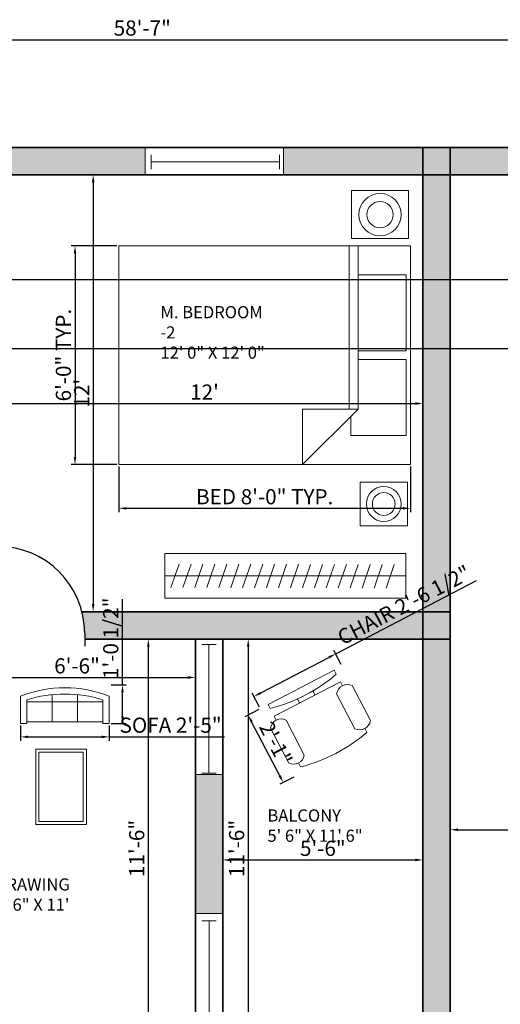
# Model space of a CAD drawing. Units: millimetres. Extents: x 2768 to 4359, y 795 to 1583.
# Tile 12 of 13: x 3930 to 4089, y 1258 to 1583. Entities that reach past the tile are written whole.
import ezdxf

# ---------------------------------------------------------------- set-up
doc = ezdxf.new("R2010")
doc.units = ezdxf.units.MM
for name, color, linetype, lineweight in [('A-ANNO-DIMS', 90, 'Continuous', 18), ('A-AREA-IDEN', 190, 'Continuous', 18), ('A-FLOR-CASE', 50, 'Continuous', 18), ('A-FLOR-CASE-PATT', 50, 'Continuous', 13), ('A-WALL-PATT', 140, 'Continuous', 9), ('doors', 10, 'Continuous', 25), ('furniture', 50, 'Continuous', 18), ('walls', 140, 'Continuous', 35), ('windows', 30, 'Continuous', 18)]:
    doc.layers.add(name, color=color, linetype=linetype, lineweight=lineweight)
doc.styles.get("Standard").update_dxf_attribs({"font": 'arial.ttf'})
doc.dimstyles.new('ISO-25', dxfattribs={"dimtxt": 5, "dimasz": 2.5, "dimexe": 1.25, "dimexo": 0.625, "dimtad": 1, "dimdec": 0, "dimlunit": 3, "dimtxsty": 'Standard', "dimcen": 2.5, "dimadec": 0, "dimazin": 0, "dimtfac": 1, "dimtdec": 0, "dimtmove": 0, "dimatfit": 3, "dimfxl": 1, "dimarcsym": 0})

# ---------------------------------------------------------------- blocks, each defined once
blk = doc.blocks.new('*U2')
for p, q in [((0, 0), (0, -6)), ((40, 0), (40, -6))]:
    blk.add_line(p, q)
blk.add_lwpolyline([(0, 0), (0, 40), (1.75, 40), (1.75, 0)], close=True)
blk.add_arc((0, 0), 40, 0, 90)
blk = doc.blocks.new('*U39')
for p, q in [((0, 4), (0, 0)), ((36, 4), (36, 0)), ((0, 2), (36, 2))]:
    blk.add_line(p, q)
blk = doc.blocks.new('Bed - Queen')
for p, q in [((0, -80.00003), (0, 0)), ((0, 0), (59.99999, 0)), ((59.99999, 0), (59.99999, -80.00003)), ((7.99999, -1.2), (28.79998, -1.2)), ((7.99999, -14.4), (7.99999, -1.2)), ((28.79998, -1.2), (28.79998, -14.4)), ((31.19999, -1.2), (51.99999, -1.2)), ((31.19999, -14.4), (31.19999, -1.2)), ((51.99999, -1.2), (51.99999, -16.4)), ((0, -14.4), (44.8, -14.4)), ((59.99999, -29.6), (44.8, -14.4)), ((44.8, -14.4), (44.8, -29.6)), ((44.8, -16.8), (0, -16.8)), ((51.99999, -16.4), (46.79936, -16.4)), ((44.8, -29.6), (59.99999, -29.6)), ((59.99999, -80.00003), (0, -80.00003))]:
    blk.add_line(p, q)
blk = doc.blocks.new('Chair - Desk')
for p, q in [((-8.5, 0), (-8.5, -1)), ((-8.5, 0), (8.5, 0)), ((8.5, 0), (8.5, -1)), ((-2, -3), (-2, -1.9355)), ((2, -1.9576), (2, -3)), ((-8.5, -3), (-8.5, -4)), ((-8.5, -3), (8.5, -3)), ((8.5, -3), (8.5, -4)), ((-10.5, -5), (-10.5, -14)), ((-6.5, -14), (-6.5, -5)), ((6.5, -5), (6.5, -14)), ((10.5, -14), (10.5, -5)), ((-8.5, -15), (-8.5, -16)), ((8.5, -15), (8.5, -16))]:
    blk.add_line(p, q)
for centre, radius, start, end in [((0, 34.625), 36.625, 256.5803, 283.4197), ((-8.5, -6.5), 2.5, 36.8699, 143.1301), ((8.5, -6.5), 2.5, 36.8699, 143.1301), ((-8.5, -12.5), 2.5, 216.8699, 323.1301), ((8.5, -12.5), 2.5, 216.8699, 323.1301), ((0, 19.625), 36.625, 256.5803, 283.4197)]:
    blk.add_arc(centre, radius, start, end)
blk = doc.blocks.new('Sofa - Roundback 7 ft.')
for p, q in [((-12.00002, -32.4421), (-12.00003, -6.5971)), ((11.99997, -32.4421), (11.99998, -6.5971)), ((-36.000027, -34), (-36.000027, -11.4696)), ((-35.999844, -13.3819), (35.9998, -13.3819)), ((35.99998, -34), (35.99998, -11.4696)), ((-36.000027, -32.4421), (35.99998, -32.4421))]:
    blk.add_line(p, q)
for points in [[(-36.000027, -34), (-42.000027, -34), (-42.000027, -8)], [(41.99998, -8), (41.99998, -34), (35.99998, -34)]]:
    blk.add_lwpolyline(points)
for centre, radius, start, end in [((0, -114.25), 114.25, 68.43141, 111.5686), ((-0.00001, -127.1968), 121.1968, 72.72033, 107.2797)]:
    blk.add_arc(centre, radius, start, end)
blk = doc.blocks.new('*D46')
at = {"layer": 'A-ANNO-DIMS', "color": 0, "lineweight": -2, "transparency": 16777216}
for p, q in [((3919.37, 1457.04), (3919.37, 1457.66)), ((4063.37, 1457.04), (4063.37, 1457.66)), ((3921.87, 1456.41), (4060.87, 1456.41))]:
    blk.add_line(p, q, dxfattribs=at)
at = {"layer": 'A-ANNO-DIMS', "color": 0, "transparency": 16777216}
for points in [[(3921.87, 1456.83), (3921.87, 1456), (3919.37, 1456.41)], [(4060.87, 1456.83), (4060.87, 1456), (4063.37, 1456.41)]]:
    blk.add_solid(points, dxfattribs=at)
at = {"layer": 'Defpoints', "color": 0, "transparency": 16777216}
for p in [(3919.37, 1456.41), (4063.37, 1456.41), (4063.37, 1456.41)]:
    blk.add_point(p, dxfattribs=at)
at = {"layer": 'A-ANNO-DIMS', "color": 0, "transparency": 16777216, "insert": (3991.37, 1459.55), "char_height": 5, "attachment_point": 5}
blk.add_mtext("12'", dxfattribs=at)
blk = doc.blocks.new('*D47')
at = {"layer": 'A-ANNO-DIMS', "color": 0, "lineweight": -2, "transparency": 16777216}
for p, q in [((3965.35, 1531.81), (3953.44, 1531.81)), ((3954.69, 1529.31), (3954.69, 1390.31)), ((3965.35, 1387.81), (3953.44, 1387.81))]:
    blk.add_line(p, q, dxfattribs=at)
at = {"layer": 'A-ANNO-DIMS', "color": 0, "transparency": 16777216}
for points in [[(3954.27, 1529.31), (3955.1, 1529.31), (3954.69, 1531.81)], [(3954.27, 1390.31), (3955.1, 1390.31), (3954.69, 1387.81)]]:
    blk.add_solid(points, dxfattribs=at)
at = {"layer": 'Defpoints', "color": 0, "transparency": 16777216}
for p in [(3965.98, 1531.81), (3954.69, 1387.81), (3965.98, 1387.81)]:
    blk.add_point(p, dxfattribs=at)
at = {"layer": 'A-ANNO-DIMS', "color": 0, "transparency": 16777216, "insert": (3951.55, 1459.81), "char_height": 5, "attachment_point": 5, "rotation": 90}
blk.add_mtext("12'", dxfattribs=at)
blk = doc.blocks.new('*D48')
at = {"layer": 'A-ANNO-DIMS', "color": 0, "lineweight": -2, "transparency": 16777216}
for p, q in [((3997.37, 1305.93), (3997.37, 1307.28)), ((3999.87, 1306.03), (4060.87, 1306.03)), ((4063.37, 1305.93), (4063.37, 1307.28))]:
    blk.add_line(p, q, dxfattribs=at)
at = {"layer": 'A-ANNO-DIMS', "color": 0, "transparency": 16777216}
for points in [[(3999.87, 1306.45), (3999.87, 1305.61), (3997.37, 1306.03)], [(4060.87, 1306.45), (4060.87, 1305.61), (4063.37, 1306.03)]]:
    blk.add_solid(points, dxfattribs=at)
at = {"layer": 'Defpoints', "color": 0, "transparency": 16777216}
for p in [(3997.37, 1305.31), (4063.37, 1306.03), (4063.37, 1305.31)]:
    blk.add_point(p, dxfattribs=at)
at = {"layer": 'A-ANNO-DIMS', "color": 0, "transparency": 16777216, "insert": (4030.37, 1309.21), "char_height": 5, "attachment_point": 5}
blk.add_mtext('5\'-6"', dxfattribs=at)
blk = doc.blocks.new('*D61')
at = {"layer": 'A-ANNO-DIMS', "color": 0, "lineweight": -2, "transparency": 16777216}
for p, q in [((4003.77, 1378.81), (4007.03, 1378.81)), ((4005.78, 1376.31), (4005.78, 1243.31)), ((4003.77, 1240.81), (4007.03, 1240.81))]:
    blk.add_line(p, q, dxfattribs=at)
at = {"layer": 'A-ANNO-DIMS', "color": 0, "transparency": 16777216}
for points in [[(4005.36, 1376.31), (4006.2, 1376.31), (4005.78, 1378.81)], [(4005.36, 1243.31), (4006.2, 1243.31), (4005.78, 1240.81)]]:
    blk.add_solid(points, dxfattribs=at)
at = {"layer": 'Defpoints', "color": 0, "transparency": 16777216}
for p in [(4003.15, 1378.81), (4003.15, 1240.81), (4005.78, 1240.81)]:
    blk.add_point(p, dxfattribs=at)
at = {"layer": 'A-ANNO-DIMS', "color": 0, "transparency": 16777216, "insert": (4002.6, 1309.81), "char_height": 5, "attachment_point": 5, "rotation": 90}
blk.add_mtext('11\'-6"', dxfattribs=at)
blk = doc.blocks.new('*D62')
at = {"layer": 'A-ANNO-DIMS', "color": 0, "lineweight": -2, "transparency": 16777216}
for p, q in [((3972.05, 1378.81), (3974.11, 1378.81)), ((3972.86, 1376.31), (3972.86, 1243.31)), ((3972.05, 1240.81), (3974.11, 1240.81))]:
    blk.add_line(p, q, dxfattribs=at)
at = {"layer": 'A-ANNO-DIMS', "color": 0, "transparency": 16777216}
for points in [[(3972.45, 1376.31), (3973.28, 1376.31), (3972.86, 1378.81)], [(3972.45, 1243.31), (3973.28, 1243.31), (3972.86, 1240.81)]]:
    blk.add_solid(points, dxfattribs=at)
at = {"layer": 'Defpoints', "color": 0, "transparency": 16777216}
for p in [(3971.42, 1378.81), (3971.42, 1240.81), (3972.86, 1240.81)]:
    blk.add_point(p, dxfattribs=at)
at = {"layer": 'A-ANNO-DIMS', "color": 0, "transparency": 16777216, "insert": (3969.69, 1309.81), "char_height": 5, "attachment_point": 5, "rotation": 90}
blk.add_mtext('11\'-6"', dxfattribs=at)
blk = doc.blocks.new('*D63')
at = {"layer": 'A-ANNO-DIMS', "color": 0, "lineweight": -2, "transparency": 16777216}
for p, q in [((3910.37, 1378.18), (3910.37, 1364.91)), ((3988.37, 1378.18), (3988.37, 1364.91)), ((3912.87, 1366.16), (3985.87, 1366.16))]:
    blk.add_line(p, q, dxfattribs=at)
at = {"layer": 'A-ANNO-DIMS', "color": 0, "transparency": 16777216}
for points in [[(3912.87, 1366.57), (3912.87, 1365.74), (3910.37, 1366.16)], [(3985.87, 1366.57), (3985.87, 1365.74), (3988.37, 1366.16)]]:
    blk.add_solid(points, dxfattribs=at)
at = {"layer": 'Defpoints', "color": 0, "transparency": 16777216}
for p in [(3910.37, 1378.81), (3988.37, 1378.81), (3988.37, 1366.16)]:
    blk.add_point(p, dxfattribs=at)
at = {"layer": 'A-ANNO-DIMS', "color": 0, "transparency": 16777216, "insert": (3949.37, 1369.33), "char_height": 5, "attachment_point": 5}
blk.add_mtext('6\'-6"', dxfattribs=at)
blk = doc.blocks.new('*D66')
at = {"layer": 'A-ANNO-DIMS', "color": 0, "lineweight": -2, "transparency": 16777216}
for p, q in [((4072.37, 1313.62), (4072.37, 1317.24)), ((4313.37, 1313.62), (4313.37, 1317.24)), ((4074.87, 1315.99), (4310.87, 1315.99))]:
    blk.add_line(p, q, dxfattribs=at)
at = {"layer": 'A-ANNO-DIMS', "color": 0, "transparency": 16777216}
for points in [[(4074.87, 1316.41), (4074.87, 1315.57), (4072.37, 1315.99)], [(4310.87, 1316.41), (4310.87, 1315.57), (4313.37, 1315.99)]]:
    blk.add_solid(points, dxfattribs=at)
at = {"layer": 'Defpoints', "color": 0, "transparency": 16777216}
for p in [(4313.37, 1315.99), (4072.37, 1312.99), (4313.37, 1312.99)]:
    blk.add_point(p, dxfattribs=at)
at = {"layer": 'A-ANNO-DIMS', "color": 0, "transparency": 16777216, "insert": (4192.87, 1319.17), "char_height": 5, "attachment_point": 5}
blk.add_mtext('20\'-1"', dxfattribs=at)
blk = doc.blocks.new('*D87')
at = {"layer": 'A-ANNO-DIMS', "color": 0, "lineweight": -2, "transparency": 16777216}
for p, q in [((4034.6, 1373.93), (4080.98, 1398.11)), ((4009.9, 1361.06), (4032.38, 1372.78)), ((4036.42, 1370.45), (4034.02, 1375.04)), ((4009.5, 1356.42), (4007.11, 1361.01))]:
    blk.add_line(p, q, dxfattribs=at)
at = {"layer": 'A-ANNO-DIMS', "color": 0, "transparency": 16777216}
for points in [[(4032.19, 1373.14), (4032.58, 1372.41), (4034.6, 1373.93)], [(4009.71, 1361.43), (4010.09, 1360.69), (4007.68, 1359.9)]]:
    blk.add_solid(points, dxfattribs=at)
at = {"layer": 'Defpoints', "color": 0, "transparency": 16777216}
for p in [(4034.6, 1373.93), (4036.7, 1369.89), (4009.79, 1355.86)]:
    blk.add_point(p, dxfattribs=at)
at = {"layer": 'A-ANNO-DIMS', "color": 0, "transparency": 16777216, "insert": (4057.42, 1389.44), "char_height": 5, "attachment_point": 5, "rotation": 27.5285}
blk.add_mtext('CHAIR 2\'-6 1/2"', dxfattribs=at)
blk = doc.blocks.new('*D88')
at = {"layer": 'A-ANNO-DIMS', "color": 0, "lineweight": -2, "transparency": 16777216}
for p, q in [((4009.23, 1355.58), (4004.64, 1353.18)), ((4016.17, 1333.76), (4006.91, 1351.54)), ((4020.81, 1333.36), (4016.22, 1330.97))]:
    blk.add_line(p, q, dxfattribs=at)
at = {"layer": 'A-ANNO-DIMS', "color": 0, "transparency": 16777216}
for points in [[(4007.28, 1351.74), (4006.54, 1351.35), (4005.75, 1353.76)], [(4016.54, 1333.95), (4015.8, 1333.57), (4017.33, 1331.54)]]:
    blk.add_solid(points, dxfattribs=at)
at = {"layer": 'Defpoints', "color": 0, "transparency": 16777216}
for p in [(4005.75, 1353.76), (4009.79, 1355.86), (4021.37, 1333.65)]:
    blk.add_point(p, dxfattribs=at)
at = {"layer": 'A-ANNO-DIMS', "color": 0, "transparency": 16777216, "insert": (4014.32, 1344.1), "char_height": 5, "attachment_point": 5, "rotation": 297.5285}
blk.add_mtext('2\'-1"', dxfattribs=at)
blk = doc.blocks.new('*D97')
at = {"layer": 'A-ANNO-DIMS', "color": 0, "lineweight": -2, "transparency": 16777216}
for p, q in [((3963.14, 1435.68), (3963.14, 1420.64)), ((4059.29, 1435.68), (4059.29, 1420.64)), ((3965.64, 1421.89), (4056.79, 1421.89))]:
    blk.add_line(p, q, dxfattribs=at)
at = {"layer": 'A-ANNO-DIMS', "color": 0, "transparency": 16777216}
for points in [[(3965.64, 1422.3), (3965.64, 1421.47), (3963.14, 1421.89)], [(4056.79, 1422.3), (4056.79, 1421.47), (4059.29, 1421.89)]]:
    blk.add_solid(points, dxfattribs=at)
at = {"layer": 'Defpoints', "color": 0, "transparency": 16777216}
for p in [(3963.14, 1436.31), (4059.29, 1436.31), (4059.29, 1421.89)]:
    blk.add_point(p, dxfattribs=at)
at = {"layer": 'A-ANNO-DIMS', "color": 0, "transparency": 16777216, "insert": (4011.21, 1425.06), "char_height": 5, "attachment_point": 5}
blk.add_mtext('BED 8\'-0" TYP.', dxfattribs=at)
blk = doc.blocks.new('*D98')
at = {"layer": 'A-ANNO-DIMS', "color": 0, "lineweight": -2, "transparency": 16777216}
for p, q in [((3962.51, 1508.42), (3947.46, 1508.42)), ((3948.71, 1505.92), (3948.71, 1438.81)), ((3962.51, 1436.31), (3947.46, 1436.31))]:
    blk.add_line(p, q, dxfattribs=at)
at = {"layer": 'A-ANNO-DIMS', "color": 0, "transparency": 16777216}
for points in [[(3948.3, 1505.92), (3949.13, 1505.92), (3948.71, 1508.42)], [(3948.3, 1438.81), (3949.13, 1438.81), (3948.71, 1436.31)]]:
    blk.add_solid(points, dxfattribs=at)
at = {"layer": 'Defpoints', "color": 0, "transparency": 16777216}
for p in [(3963.14, 1508.42), (3948.71, 1436.31), (3963.14, 1436.31)]:
    blk.add_point(p, dxfattribs=at)
at = {"layer": 'A-ANNO-DIMS', "color": 0, "transparency": 16777216, "insert": (3945.53, 1472.37), "char_height": 5, "attachment_point": 5, "rotation": 90}
blk.add_mtext('6\'-0" TYP.', dxfattribs=at)
blk = doc.blocks.new('*D107')
at = {"layer": 'A-ANNO-DIMS', "color": 0, "lineweight": -2, "transparency": 16777216}
for p, q in [((3930.77, 1350.33), (3930.77, 1345.33)), ((3959.97, 1350.33), (3959.97, 1345.33)), ((3933.27, 1346.58), (3957.47, 1346.58)), ((3959.97, 1346.58), (3997.95, 1346.58))]:
    blk.add_line(p, q, dxfattribs=at)
at = {"layer": 'A-ANNO-DIMS', "color": 0, "transparency": 16777216}
for points in [[(3933.27, 1347), (3933.27, 1346.16), (3930.77, 1346.58)], [(3957.47, 1347), (3957.47, 1346.16), (3959.97, 1346.58)]]:
    blk.add_solid(points, dxfattribs=at)
at = {"layer": 'Defpoints', "color": 0, "transparency": 16777216}
for p in [(3930.77, 1350.96), (3959.97, 1350.96), (3959.97, 1346.58)]:
    blk.add_point(p, dxfattribs=at)
at = {"layer": 'A-ANNO-DIMS', "color": 0, "transparency": 16777216, "insert": (3980.21, 1349.79), "char_height": 5, "attachment_point": 5}
blk.add_mtext('SOFA 2\'-5"', dxfattribs=at)
blk = doc.blocks.new('*D108')
at = {"layer": 'A-ANNO-DIMS', "color": 0, "lineweight": -2, "transparency": 16777216}
for p, q in [((3964.35, 1363.71), (3964.35, 1391.93)), ((3960.6, 1363.71), (3965.6, 1363.71)), ((3964.35, 1353.46), (3964.35, 1361.21)), ((3960.6, 1350.96), (3965.6, 1350.96))]:
    blk.add_line(p, q, dxfattribs=at)
at = {"layer": 'A-ANNO-DIMS', "color": 0, "transparency": 16777216}
for points in [[(3963.94, 1361.21), (3964.77, 1361.21), (3964.35, 1363.71)], [(3963.94, 1353.46), (3964.77, 1353.46), (3964.35, 1350.96)]]:
    blk.add_solid(points, dxfattribs=at)
at = {"layer": 'Defpoints', "color": 0, "transparency": 16777216}
for p in [(3959.97, 1363.71), (3964.35, 1363.71), (3959.97, 1350.96)]:
    blk.add_point(p, dxfattribs=at)
at = {"layer": 'A-ANNO-DIMS', "color": 0, "transparency": 16777216, "insert": (3961.14, 1379.07), "char_height": 5, "attachment_point": 5, "rotation": 90}
blk.add_mtext('1\'-0 1/2"', dxfattribs=at)
blk = doc.blocks.new('*D128')
at = {"layer": 'A-ANNO-DIMS', "color": 0, "lineweight": -2, "transparency": 16777216}
for p, q in [((3619.37, 1541.43), (3619.37, 1577.56)), ((4322.37, 1541.43), (4322.37, 1577.56)), ((3621.87, 1576.31), (4319.87, 1576.31))]:
    blk.add_line(p, q, dxfattribs=at)
at = {"layer": 'A-ANNO-DIMS', "color": 0, "transparency": 16777216}
for points in [[(3621.87, 1576.72), (3621.87, 1575.89), (3619.37, 1576.31)], [(4319.87, 1576.72), (4319.87, 1575.89), (4322.37, 1576.31)]]:
    blk.add_solid(points, dxfattribs=at)
at = {"layer": 'Defpoints', "color": 0, "transparency": 16777216}
for p in [(4322.37, 1576.31), (3619.37, 1540.81), (4322.37, 1540.81)]:
    blk.add_point(p, dxfattribs=at)
at = {"layer": 'A-ANNO-DIMS', "color": 0, "transparency": 16777216, "insert": (3970.87, 1579.49), "char_height": 5, "attachment_point": 5}
blk.add_mtext('58\'-7"', dxfattribs=at)
blk = doc.blocks.new('*D136')
at = {"layer": 'A-ANNO-DIMS', "color": 0, "lineweight": -2, "transparency": 16777216}
for p, q in [((3919.99, 1497.31), (4359.12, 1497.31)), ((4357.87, 1477.05), (4357.87, 1494.81)), ((3919.99, 1474.55), (4359.12, 1474.55))]:
    blk.add_line(p, q, dxfattribs=at)
at = {"layer": 'A-ANNO-DIMS', "color": 0, "transparency": 16777216}
for points in [[(4357.45, 1494.81), (4358.28, 1494.81), (4357.87, 1497.31)], [(4357.45, 1477.05), (4358.28, 1477.05), (4357.87, 1474.55)]]:
    blk.add_solid(points, dxfattribs=at)
at = {"layer": 'Defpoints', "color": 0, "transparency": 16777216}
for p in [(3919.37, 1497.31), (4357.87, 1497.31), (3919.37, 1474.55)]:
    blk.add_point(p, dxfattribs=at)
at = {"layer": 'A-ANNO-DIMS', "color": 0, "transparency": 16777216, "insert": (4354.73, 1485.93), "char_height": 5, "attachment_point": 5, "rotation": 90}
blk.add_mtext('1\'-11"', dxfattribs=at)

msp = doc.modelspace()

# ---------------------------------------------------------------- hatches: boundary and pattern name
at = {"layer": 'A-FLOR-CASE-PATT'}
h = msp.add_hatch(dxfattribs=at)
h.set_pattern_fill('ANSI31', color=256, scale=1.173362, angle=25.981, style=0)
h.paths.add_polyline_path([(4056.48, 1403.35), (4053.81, 1395.61), (3979, 1395.79), (3981.67, 1403.54)])
at = {"layer": 'A-WALL-PATT'}
h = msp.add_hatch(color=256, dxfattribs=at)
h.dxf.hatch_style = 1
h.paths.add_polyline_path([(3666.8, 1540.81), (3628.37, 1540.81), (3628.37, 1531.81), (3666.8, 1531.81)])
h.paths.add_polyline_path([(3628.37, 1540.81), (3619.37, 1540.81), (3619.37, 1531.81), (3628.37, 1531.81)])
h.paths.add_polyline_path([(3628.37, 1531.81), (3619.37, 1531.81), (3619.37, 1387.81), (3628.37, 1387.81)])
h.paths.add_polyline_path([(3772.37, 1540.81), (3710.62, 1540.81), (3710.62, 1531.81), (3772.37, 1531.81)])
h.paths.add_polyline_path([(3796.31, 1540.81), (3781.37, 1540.81), (3781.37, 1531.81), (3796.31, 1531.81)])
h.paths.add_polyline_path([(3781.37, 1540.81), (3772.37, 1540.81), (3772.37, 1531.81), (3781.37, 1531.81)])
h.paths.add_polyline_path([(3781.37, 1531.81), (3772.37, 1531.81), (3772.37, 1493.05), (3773.51, 1493.08), (3781.37, 1493.27)])
h.paths.add_polyline_path([(3841.37, 1540.81), (3822.12, 1540.81), (3822.12, 1531.81), (3841.37, 1531.81)])
h.paths.add_polyline_path([(3867.29, 1540.81), (3850.37, 1540.81), (3850.37, 1531.81), (3867.29, 1531.81)])
h.paths.add_polyline_path([(3850.37, 1540.81), (3841.37, 1540.81), (3841.37, 1531.81), (3850.37, 1531.81)])
h.paths.add_polyline_path([(3850.37, 1531.81), (3841.37, 1531.81), (3841.37, 1435.81), (3850.37, 1435.81)])
h.paths.add_polyline_path([(3919.37, 1531.81), (3910.37, 1531.81), (3910.37, 1495.39, -0.097322), (3918.93, 1497.3), (3919.37, 1497.31)])
h.paths.add_polyline_path([(3919.37, 1540.81), (3910.37, 1540.81), (3910.37, 1531.81), (3919.37, 1531.81)])
h.paths.add_polyline_path([(3910.37, 1540.81), (3893.19, 1540.81), (3893.19, 1531.81), (3910.37, 1531.81)])
h.paths.add_polyline_path([(3971.85, 1540.81), (3919.37, 1540.81), (3919.37, 1531.81), (3971.85, 1531.81)])
h.paths.add_polyline_path([(4063.37, 1540.81), (4017.44, 1540.81), (4017.44, 1531.81), (4063.37, 1531.81)])
h.paths.add_polyline_path([(4072.37, 1531.81), (4063.37, 1531.81), (4063.37, 1387.81), (4072.37, 1387.81)])
h.paths.add_polyline_path([(4072.37, 1378.81), (4063.37, 1378.81), (4063.37, 1240.81), (4072.37, 1240.81)])
h.paths.add_polyline_path([(4072.37, 1387.81), (4063.37, 1387.81), (4063.37, 1378.81), (4072.37, 1378.81)])
h.paths.add_polyline_path([(3919.37, 1387.81), (3910.37, 1387.81), (3910.37, 1378.81), (3919.37, 1378.81)])
h.paths.add_polyline_path([(3919.37, 1392.95, -0.05459), (3913.18, 1392.28), (3910.37, 1392.28), (3910.37, 1387.81), (3919.37, 1387.81)])
h.paths.add_polyline_path([(3919.37, 1474.55), (3910.37, 1474.32), (3910.37, 1435.81), (3919.37, 1435.81)])
h.paths.add_polyline_path([(3919.37, 1435.81), (3910.37, 1435.81), (3910.37, 1426.81), (3919.37, 1426.81)])
h.paths.add_polyline_path([(3910.37, 1435.81), (3850.37, 1435.81), (3850.37, 1426.81), (3910.37, 1426.81)])
h.paths.add_polyline_path([(3919.37, 1426.81), (3910.37, 1426.81), (3910.37, 1420.86), (3913.18, 1420.86), (3919.37, 1420.86)])
h.paths.add_polyline_path([(3850.37, 1435.81), (3841.37, 1435.81), (3841.37, 1426.81), (3850.37, 1426.81)])
h.paths.add_polyline_path([(3841.37, 1435.81), (3781.37, 1435.81), (3781.37, 1426.81), (3841.37, 1426.81)])
h.paths.add_polyline_path([(3781.37, 1435.81), (3772.37, 1435.81), (3772.37, 1426.81), (3781.37, 1426.81)])
h.paths.add_polyline_path([(3781.37, 1426.81), (3772.37, 1426.81), (3772.37, 1420.59, -0.050492), (3778.09, 1421.17), (3781.37, 1421.17)])
h.paths.add_polyline_path([(3781.37, 1471.72, -0.082137), (3774.07, 1470.33), (3772.37, 1470.29), (3772.37, 1435.81), (3781.37, 1435.81)])
h.paths.add_polyline_path([(3628.37, 1387.81), (3619.37, 1387.81), (3619.37, 1378.81), (3628.37, 1378.81)])
h.paths.add_polyline_path([(3628.37, 1378.81), (3619.37, 1378.81), (3619.37, 1346.39), (3622.95, 1346.39), (3628.37, 1346.39)])
h.paths.add_polyline_path([(3781.37, 1387.81), (3772.37, 1387.81), (3772.37, 1378.81), (3781.37, 1378.81)])
h.paths.add_polyline_path([(3781.37, 1392.59), (3778.09, 1392.59), (3772.37, 1392.59), (3772.37, 1387.81), (3781.37, 1387.81)])
h.paths.add_polyline_path([(3628.37, 1318.32, -0.047705), (3622.95, 1317.81), (3619.37, 1317.81), (3619.37, 1221.81), (3628.37, 1221.81)])
h.paths.add_polyline_path([(3628.37, 1221.81), (3619.37, 1221.81), (3619.37, 1212.81), (3628.37, 1212.81)])
h.paths.add_polyline_path([(3827.37, 1221.81), (3628.37, 1221.81), (3628.37, 1212.81), (3827.37, 1212.81)])
h.paths.add_polyline_path([(3628.37, 1212.81), (3619.37, 1212.81), (3619.37, 1116.81), (3628.37, 1116.81)])
h.paths.add_polyline_path([(3836.37, 1221.81), (3827.37, 1221.81), (3827.37, 1212.81), (3836.37, 1212.81)])
h.paths.add_polyline_path([(3628.37, 1107.81), (3619.37, 1107.81), (3619.37, 1047.81), (3628.37, 1047.81)])
h.paths.add_polyline_path([(3628.37, 1116.81), (3619.37, 1116.81), (3619.37, 1107.81), (3628.37, 1107.81)])
h.paths.add_polyline_path([(3836.37, 1155.81), (3827.37, 1155.81), (3827.37, 1116.81), (3836.37, 1116.81)])
h.paths.add_polyline_path([(3836.37, 1116.81), (3827.37, 1116.81), (3827.37, 1107.81), (3836.37, 1107.81)])
h.paths.add_polyline_path([(3836.37, 1107.81), (3827.37, 1107.81), (3827.37, 1047.81), (3836.37, 1047.81)])
h.paths.add_polyline_path([(3827.37, 1047.37), (3827.37, 1047.81), (3739.96, 1047.81), (3739.96, 1038.81), (3827.37, 1038.81)])
h.paths.add_polyline_path([(3836.37, 1047.37), (3836.37, 1047.81), (3827.37, 1047.81), (3827.37, 1047.37), (3827.37, 1038.81), (3836.37, 1038.81)])
h.paths.add_polyline_path([(3695.08, 1047.81), (3628.37, 1047.81), (3628.37, 1038.81), (3695.08, 1038.81)])
h.paths.add_polyline_path([(3628.37, 1047.81), (3619.37, 1047.81), (3619.37, 1038.81), (3628.37, 1038.81)])
h.paths.add_polyline_path([(3850.59, 1047.81), (3836.37, 1047.81), (3836.37, 1047.37), (3836.37, 1038.81), (3850.59, 1038.81)])
h.paths.add_polyline_path([(3896.37, 1047.37), (3896.37, 1047.81), (3876.26, 1047.81), (3876.26, 1038.81), (3896.37, 1038.81)])
h.paths.add_polyline_path([(3905.37, 1109.65), (3903.46, 1109.6), (3896.37, 1109.43), (3896.37, 1047.81), (3905.37, 1047.81)])
h.paths.add_polyline_path([(3905.37, 1047.81), (3896.37, 1047.81), (3896.37, 1047.37), (3896.37, 1038.81), (3905.37, 1038.81)])
h.paths.add_polyline_path([(4063.37, 1047.81), (3905.37, 1047.81), (3905.37, 1038.81), (4063.37, 1038.81)])
h.paths.add_polyline_path([(4072.37, 1137.28), (4063.37, 1137.28), (4063.37, 1047.81), (4072.37, 1047.81)])
h.paths.add_polyline_path([(4072.37, 1231.81), (4063.37, 1231.81), (4063.37, 1182.55), (4072.37, 1182.55)])
h.paths.add_polyline_path([(4072.37, 1240.81), (4063.37, 1240.81), (4063.37, 1231.81), (4072.37, 1231.81)])
h.paths.add_polyline_path([(4072.37, 1047.81), (4063.37, 1047.81), (4063.37, 1038.81), (4072.37, 1038.81)])
h.paths.add_polyline_path([(3905.37, 1231.81), (3896.37, 1231.81), (3896.37, 1164.81), (3905.37, 1164.81)])
h.paths.add_polyline_path([(3905.37, 1240.81), (3896.37, 1240.81), (3896.37, 1231.81), (3905.37, 1231.81)])
h.paths.add_polyline_path([(3910.61, 1237.57), (3910.61, 1240.81), (3905.37, 1240.81), (3905.37, 1231.81), (3911.2, 1231.81, -0.050754)])
h.paths.add_polyline_path([(3988.37, 1240.81), (3939.19, 1240.81), (3939.19, 1237.57), (3939.19, 1231.81), (3988.37, 1231.81)])
h.paths.add_polyline_path([(3997.37, 1240.81), (3988.37, 1240.81), (3988.37, 1231.81), (3997.37, 1231.81)])
h.paths.add_polyline_path([(4063.37, 1240.81), (3997.37, 1240.81), (3997.37, 1231.81), (4063.37, 1231.81)])
h.paths.add_polyline_path([(3997.37, 1334.21), (3988.37, 1334.21), (3988.37, 1288.44), (3997.37, 1288.44)])
h.paths.add_polyline_path([(3896.37, 1164.81), (3836.37, 1164.81), (3836.37, 1155.81), (3896.37, 1155.81)])
h.paths.add_polyline_path([(3836.37, 1164.81), (3827.37, 1164.81), (3827.37, 1155.81), (3836.37, 1155.81)])
h.paths.add_polyline_path([(3905.37, 1164.81), (3896.37, 1164.81), (3896.37, 1155.81), (3905.37, 1155.81)])
h.paths.add_polyline_path([(3905.37, 1155.81), (3896.37, 1155.81), (3896.37, 1131.22, -0.073168), (3902.89, 1132.35), (3905.37, 1132.41)])
edge = h.paths.add_edge_path()
edge.add_line((3951.89, 1380.74), (3951.89, 1378.81))
edge.add_line((3951.89, 1378.81), (4063.37, 1378.81))
edge.add_line((4063.37, 1378.81), (4063.37, 1387.81))
edge.add_line((4063.37, 1387.81), (3951, 1387.81))
edge.add_arc((3923.31, 1380.74), 28.58, 0, 14.3236, ccw=False)
h.paths.add_polyline_path([(3923.31, 1378.81), (3923.31, 1387.81), (3919.37, 1387.81), (3919.37, 1378.81)])
edge = h.paths.add_edge_path()
edge.add_arc((3775.74, 1114.53), 22.75, 187.4686, 197.1843)
edge.add_line((3754, 1107.81), (3628.37, 1107.81))
edge.add_line((3628.37, 1107.81), (3628.37, 1116.81))
edge.add_line((3628.37, 1116.81), (3752.42, 1116.81))
edge.add_arc((3775.17, 1117.41), 22.75, 181.5276, 194.8757)
h.paths.add_polyline_path([(3775.68, 1116.81), (3775.91, 1107.81), (3827.37, 1107.81), (3827.37, 1116.81)])
h = msp.add_hatch(color=256, dxfattribs=at)
h.dxf.hatch_style = 1
h.paths.add_polyline_path([(4313.37, 1540.81), (4072.37, 1540.81), (4072.37, 1531.81), (4313.37, 1531.81)])
h.paths.add_polyline_path([(4072.37, 1540.81), (4063.37, 1540.81), (4063.37, 1531.81), (4072.37, 1531.81)])
h.paths.add_polyline_path([(4322.37, 1540.81), (4313.37, 1540.81), (4313.37, 1531.81), (4322.37, 1531.81)])
h.paths.add_polyline_path([(4322.37, 1531.81), (4313.37, 1531.81), (4313.37, 1378.81), (4313.37, 1047.81), (4322.37, 1047.81), (4322.37, 1378.81)])
h.paths.add_polyline_path([(4313.37, 1047.81), (4072.37, 1047.81), (4072.37, 1038.81), (4313.37, 1038.81)])

# ---------------------------------------------------------------- linework, layer by layer
at = {"layer": 'A-FLOR-CASE'}
msp.add_line((3978.32, 1399.67), (4057.67, 1399.67), dxfattribs=at)
msp.add_lwpolyline([(4057.67, 1392.29), (3978.32, 1392.29), (3978.32, 1407.05), (4057.67, 1407.05)], close=True, dxfattribs=at)
at = {"layer": 'furniture'}
for points in [[(4058.6, 1510.75), (4039.86, 1510.75), (4039.86, 1526.56), (4058.6, 1526.56)], [(4058.27, 1430.5), (4042.64, 1430.5), (4042.64, 1416.14), (4058.27, 1416.14)], [(3935.79, 1342.54), (3952.44, 1342.54), (3952.44, 1317.68), (3935.79, 1317.68)], [(3936.79, 1341.54), (3951.44, 1341.54), (3951.44, 1318.68), (3936.79, 1318.68)]]:
    msp.add_lwpolyline(points, close=True, dxfattribs=at)
for centre, radius in [((4049.23, 1518.65), 6.98), ((4049.23, 1518.65), 4.33), ((4050.45, 1423.32), 5.74), ((4050.45, 1423.32), 3.76)]:
    msp.add_circle(centre, radius, dxfattribs=at)
at = {"layer": 'walls'}
for p, q in [((3619.37, 1540.81), (4322.37, 1540.81)), ((4063.37, 1540.81), (4063.37, 1378.81)), ((4072.37, 1540.81), (4072.37, 1378.81)), ((3619.37, 1531.81), (4322.37, 1531.81)), ((3951, 1387.81), (4072.37, 1387.81)), ((3951.89, 1378.81), (4072.37, 1378.81)), ((3988.37, 1378.81), (3988.37, 1231.81)), ((3997.37, 1378.81), (3997.37, 1231.81)), ((4063.37, 1378.81), (4063.37, 1007.81)), ((4072.37, 1378.81), (4072.37, 1007.81))]:
    msp.add_line(p, q, dxfattribs=at)
at = {"layer": 'windows'}
for p, q in [((3971.85, 1540.81), (3971.85, 1531.81)), ((4017.44, 1540.81), (4017.44, 1531.81)), ((3988.37, 1334.21), (3997.37, 1334.21)), ((3997.37, 1288.44), (3988.37, 1288.44))]:
    msp.add_line(p, q, dxfattribs=at)

# ---------------------------------------------------------------- block references
at = {"layer": 'doors', "xscale": 0.7144929449846577, "yscale": 0.7144929449846577, "zscale": 0.7144929449846577}
msp.add_blockref('*U2', (3923.31, 1380.74), dxfattribs=at)
at = {"layer": 'furniture'}
for name, p, xscale, yscale, zscale, rotation in [('Bed - Queen', (4059.29, 1508.42), 1.201893325172568, 1.201893325172568, 1.201893325172568, 270), ('Chair - Desk', (4023.25, 1362.88), 1.445350634619206, 1.445350634619206, 1.445350634619206, 27.52852573857865)]:
    msp.add_blockref(name, p, dxfattribs=dict(at, xscale=xscale, yscale=yscale, zscale=zscale, rotation=rotation))
at = {"layer": 'furniture', "xscale": 0.3476841025892543, "yscale": 0.3476841025892543, "zscale": 0.3476841025892543}
msp.add_blockref('Sofa - Roundback 7 ft.', (3945.37, 1362.78), dxfattribs=at)
at = {"layer": 'windows', "xscale": 1.175999919670228, "yscale": 1.175999919670228, "zscale": 1.175999919670228}
msp.add_blockref('*U39', (3973.75, 1533.67), dxfattribs=at)
at = {"layer": 'windows', "xscale": 1.175999919670228, "yscale": 1.175999919670228, "zscale": 1.175999919670228, "rotation": 270}
for p in [(3990.49, 1376.98), (3990.51, 1286.01)]:
    msp.add_blockref('*U39', p, dxfattribs=at)

# ---------------------------------------------------------------- texts
at = {"layer": 'A-AREA-IDEN', "char_height": 4, "attachment_point": 1}
for s, width, insert in [('M. BEDROOM -2\\P12\' 0" X 12\' 0"', 35.2904, (3976.86, 1488.52)), ('BALCONY \\P5\' 6" X 11\' 6"', 44.2426, (4012.11, 1322.68)), ('DRAWING \\P6\' 6" X 11\' 6"', 29.6052, (3922.36, 1299.96))]:
    msp.add_mtext_dynamic_manual_height_columns(s, width=width, gutter_width=12.5, heights=[0], dxfattribs=dict(at, insert=insert))

# ---------------------------------------------------------------- dimensions: what is measured, and where the dimension line sits
at = {"layer": 'A-ANNO-DIMS'}
for base, p1, p2, override, picture, middle in [((4322.37, 1576.31), (3619.37, 1540.81), (4322.37, 1540.81), {"dimdec": 1, "dimlfac": 1, "dimrnd": 0, "dimzin": 1, "dimdsep": 46, "dimlunit": 4, "dimfrac": 2}, '*D128', (3970.87, 1579.49)), ((4063.37, 1456.41), (3919.37, 1456.41), (4063.37, 1456.41), {"dimclrd": 0, "dimclre": 0, "dimclrt": 0}, '*D46', (3991.37, 1459.55)), ((3988.37, 1366.16), (3910.37, 1378.81), (3988.37, 1378.81), {"dimclrd": 0, "dimclre": 0, "dimclrt": 0}, '*D63', (3949.37, 1369.33)), ((4313.37, 1315.99), (4072.37, 1312.99), (4313.37, 1312.99), {"dimclrd": 0, "dimclre": 0, "dimclrt": 0}, '*D66', (4192.87, 1319.17)), ((4063.37, 1306.03), (3997.37, 1305.31), (4063.37, 1305.31), {"dimclrd": 0, "dimclre": 0, "dimclrt": 0}, '*D48', (4030.37, 1309.21))]:
    dim = msp.add_linear_dim(base=base, p1=p1, p2=p2, dimstyle='ISO-25', override=override, dxfattribs=at)
    dim.commit()
    dim.dimension.update_dxf_attribs({"geometry": picture, "text_midpoint": middle})
for base, p1, p2, angle, override, picture, middle in [((3954.69, 1387.81), (3965.98, 1531.81), (3965.98, 1387.81), 90, {"dimclrd": 0, "dimclre": 0, "dimclrt": 0}, '*D47', (3951.55, 1459.81)), ((4357.87, 1497.31), (3919.37, 1474.55), (3919.37, 1497.31), 90, {"dimdec": 1, "dimlfac": 1, "dimrnd": 0, "dimzin": 1, "dimdsep": 46, "dimlunit": 4, "dimfrac": 2}, '*D136', (4354.73, 1485.93)), ((3964.3518, 1363.7077), (3959.9709, 1350.9593), (3959.9709, 1363.7077), 90, {"dimdec": 1, "dimlfac": 1, "dimrnd": 0, "dimzin": 1, "dimdsep": 46, "dimlunit": 4, "dimfrac": 2}, '*D108', (3961.1415, 1379.0684)), ((3972.86, 1240.81), (3971.42, 1378.81), (3971.42, 1240.81), 90, {"dimclrd": 0, "dimclre": 0, "dimclrt": 0}, '*D62', (3969.69, 1309.81)), ((4005.78, 1240.81), (4003.15, 1378.81), (4003.15, 1240.81), 90, {"dimclrd": 0, "dimclre": 0, "dimclrt": 0}, '*D61', (4002.6, 1309.81)), ((4005.7507, 1353.7604), (4021.3672, 1333.6483), (4009.7881, 1355.8646), 117.5285, {"dimdec": 1, "dimlfac": 1, "dimrnd": 0, "dimzin": 1, "dimdsep": 46, "dimlunit": 4, "dimfrac": 2}, '*D88', (4014.3205, 1344.1013))]:
    dim = msp.add_linear_dim(base=base, p1=p1, p2=p2, angle=angle, dimstyle='ISO-25', override=override, dxfattribs=at)
    dim.commit()
    dim.dimension.update_dxf_attribs({"geometry": picture, "text_midpoint": middle})
for base, p1, p2, angle, text, picture, middle in [((3948.71, 1436.31), (3963.14, 1508.42), (3963.14, 1436.31), 270, '<> TYP.', '*D98', (3945.53, 1472.37)), ((4034.5997, 1373.9306), (4009.7881, 1355.8646), (4036.7039, 1369.8932), 27.5285, 'CHAIR <>', '*D87', (4057.4169, 1389.4431))]:
    dim = msp.add_linear_dim(base=base, p1=p1, p2=p2, angle=angle, text=text, dimstyle='ISO-25', override={"dimdec": 1, "dimlfac": 1, "dimrnd": 0, "dimzin": 1, "dimdsep": 46, "dimlunit": 4, "dimfrac": 2}, dxfattribs=at)
    dim.commit()
    dim.dimension.update_dxf_attribs({"geometry": picture, "text_midpoint": middle})
for base, p1, p2, text, picture, middle in [((4059.2869, 1421.8871), (3963.1354, 1436.3098), (4059.2869, 1436.3098), 'BED <> TYP.', '*D97', (4011.2111, 1425.0649)), ((3959.97, 1346.58), (3930.77, 1350.96), (3959.97, 1350.96), 'SOFA <>', '*D107', (3980.21, 1349.79))]:
    dim = msp.add_linear_dim(base=base, p1=p1, p2=p2, text=text, dimstyle='ISO-25', override={"dimdec": 1, "dimlfac": 1, "dimrnd": 0, "dimzin": 1, "dimdsep": 46, "dimlunit": 4, "dimfrac": 2}, dxfattribs=at)
    dim.commit()
    dim.dimension.update_dxf_attribs({"geometry": picture, "text_midpoint": middle})

doc.saveas('drawing.dxf')
